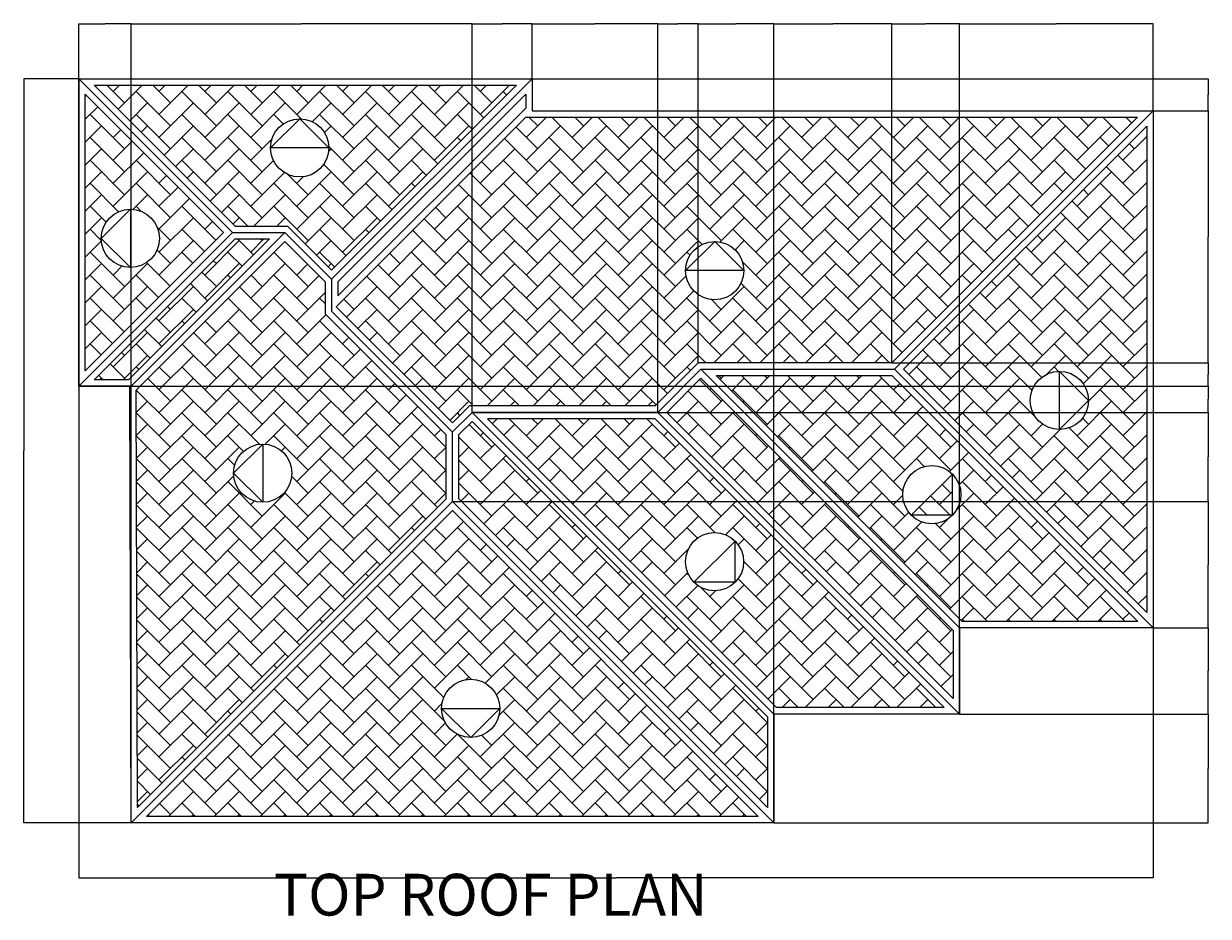
# Model space of a CAD drawing. Units: millimetres. Extents: x 19292 to 100733, y 12374 to 26974.
# Tile 23 of 24: x 60952 to 75784, y 12374 to 23551. Entities that reach past the tile are written whole.
import ezdxf

# ---------------------------------------------------------------- set-up
doc = ezdxf.new("R2010")
doc.units = ezdxf.units.MM
for name, color, linetype, lineweight in [('A-ANNO-DIMS', 2, 'Continuous', 18), ('A-ANNO-SYMB', 2, 'Continuous', 18), ('A-ANNO-TEXT', 7, 'Continuous', 35), ('A-ROOF', 6, 'Continuous', 25), ('A-ROOF-PATT', 8, 'Continuous', 13)]:
    doc.layers.add(name, color=color, linetype=linetype, lineweight=lineweight)
doc.styles.get("Standard").update_dxf_attribs({"font": 'arial.ttf'})
doc.dimstyles.get("Standard").update_dxf_attribs({"dimtxt": 0.18, "dimasz": 0.18, "dimexe": 0.18, "dimexo": 0.0625, "dimgap": 0.09, "dimtad": 0, "dimtih": 1, "dimtoh": 1, "dimdec": 4, "dimzin": 0, "dimdsep": 46, "dimtxsty": 'Standard', "dimcen": 0.09, "dimadec": 0, "dimazin": 0, "dimtfac": 1, "dimtdec": 4, "dimtofl": 0, "dimtmove": 0, "dimatfit": 3, "dimfxl": 1, "dimtolj": 1, "dimtzin": 0, "dimarcsym": 0})

# ---------------------------------------------------------------- blocks, each defined once
blk = doc.blocks.new('ROOF-SLOPE-SYMB')
for p, q in [((364.4880056519105, 728.9755004564394), (0.0002616674464662, 364.4877564719863)), ((364.4880056519105, 728.9755004564394), (728.9757496363599, 364.4877564719791)), ((728.9757496363673, 364.4877564719645), (0.0002616674464662, 364.4877564719863))]:
    blk.add_line(p, q)
blk.add_circle((364.4880056519032, 364.4877564719827), 364.4877439844593)
blk = doc.blocks.new('*D122')
at = {"layer": 'A-ANNO-DIMS', "color": 0, "lineweight": -2, "transparency": 16777216}
for p, q in [((61642.733569, 22860.787437), (61642.733569, 23550.904937)), ((61642.913569, 23550.724937), (61969.68047341132, 23550.724937)), ((62297.235768, 23550.724937), (61970.46886358869, 23550.724937)), ((62297.415768, 13544.0551), (62297.415768, 23550.904937))]:
    blk.add_line(p, q, dxfattribs=at)
at = {"layer": 'A-ANNO-DIMS', "color": 0, "transparency": 16777216}
for points in [[(61642.913569, 23550.754937), (61642.913569, 23550.694937), (61642.733569, 23550.724937)], [(62297.235768, 23550.754937), (62297.235768, 23550.694937), (62297.415768, 23550.724937)]]:
    blk.add_solid(points, dxfattribs=at)
at = {"layer": 'Defpoints', "color": 0, "transparency": 16777216}
for p in [(62297.415768, 23550.724937), (61642.733569, 22860.724937), (62297.415768, 13543.9926)]:
    blk.add_point(p, dxfattribs=at)
at = {"layer": 'A-ANNO-DIMS', "color": 0, "transparency": 16777216, "insert": (61970.0746685, 23550.724937), "char_height": 0.18, "attachment_point": 5}
blk.add_mtext('\\A1;654.7', dxfattribs=at)
blk = doc.blocks.new('*D123')
at = {"layer": 'A-ANNO-DIMS', "color": 0, "lineweight": -2, "transparency": 16777216}
for p, q in [((62297.415768, 13544.0551), (62297.415768, 23550.904937)), ((62297.595768, 23550.724937), (64431.20193955525, 23550.724937)), ((66565.53326800001, 23550.724937), (64431.92709644476, 23550.724937)), ((66565.713268, 18684.151922), (66565.713268, 23550.904937))]:
    blk.add_line(p, q, dxfattribs=at)
at = {"layer": 'A-ANNO-DIMS', "color": 0, "transparency": 16777216}
for points in [[(62297.595768, 23550.754937), (62297.595768, 23550.694937), (62297.415768, 23550.724937)], [(66565.53326800001, 23550.754937), (66565.53326800001, 23550.694937), (66565.713268, 23550.724937)]]:
    blk.add_solid(points, dxfattribs=at)
at = {"layer": 'Defpoints', "color": 0, "transparency": 16777216}
for p in [(66565.713268, 23550.724937), (66565.713268, 18684.089422), (62297.415768, 13543.9926)]:
    blk.add_point(p, dxfattribs=at)
at = {"layer": 'A-ANNO-DIMS', "color": 0, "transparency": 16777216, "insert": (64431.56451800001, 23550.724937), "char_height": 0.18, "attachment_point": 5}
blk.add_mtext('\\A1;4268', dxfattribs=at)
blk = doc.blocks.new('*D124')
at = {"layer": 'A-ANNO-DIMS', "color": 0, "lineweight": -2, "transparency": 16777216}
for p, q in [((66565.713268, 18684.151922), (66565.713268, 23550.904937)), ((66565.893268, 23550.724937), (66941.43622886836, 23550.724937)), ((67317.55356900001, 23550.724937), (66942.01060813166, 23550.724937)), ((67317.733569, 22860.787437), (67317.733569, 23550.904937))]:
    blk.add_line(p, q, dxfattribs=at)
at = {"layer": 'A-ANNO-DIMS', "color": 0, "transparency": 16777216}
for points in [[(66565.893268, 23550.754937), (66565.893268, 23550.694937), (66565.713268, 23550.724937)], [(67317.55356900001, 23550.754937), (67317.55356900001, 23550.694937), (67317.733569, 23550.724937)]]:
    blk.add_solid(points, dxfattribs=at)
at = {"layer": 'Defpoints', "color": 0, "transparency": 16777216}
for p in [(67317.733569, 23550.724937), (67317.733569, 22860.724937), (66565.713268, 18684.089422)]:
    blk.add_point(p, dxfattribs=at)
at = {"layer": 'A-ANNO-DIMS', "color": 0, "transparency": 16777216, "insert": (66941.72341850001, 23550.724937), "char_height": 0.18, "attachment_point": 5}
blk.add_mtext('\\A1;752', dxfattribs=at)
blk = doc.blocks.new('*D125')
at = {"layer": 'A-ANNO-DIMS', "color": 0, "lineweight": -2, "transparency": 16777216}
for p, q in [((67317.733569, 22860.787437), (67317.733569, 23550.904937)), ((67317.913569, 23550.724937), (68103.69878993586, 23550.724937)), ((68890.394693, 23550.724937), (68104.60947206413, 23550.724937)), ((68890.574693, 18684.151922), (68890.574693, 23550.904937))]:
    blk.add_line(p, q, dxfattribs=at)
at = {"layer": 'A-ANNO-DIMS', "color": 0, "transparency": 16777216}
for points in [[(67317.913569, 23550.754937), (67317.913569, 23550.694937), (67317.733569, 23550.724937)], [(68890.394693, 23550.754937), (68890.394693, 23550.694937), (68890.574693, 23550.724937)]]:
    blk.add_solid(points, dxfattribs=at)
at = {"layer": 'Defpoints', "color": 0, "transparency": 16777216}
for p in [(68890.574693, 23550.724937), (67317.733569, 22860.724937), (68890.574693, 18684.089422)]:
    blk.add_point(p, dxfattribs=at)
at = {"layer": 'A-ANNO-DIMS', "color": 0, "transparency": 16777216, "insert": (68104.154131, 23550.724937), "char_height": 0.18, "attachment_point": 5}
blk.add_mtext('\\A1;1572.8', dxfattribs=at)
blk = doc.blocks.new('*D126')
at = {"layer": 'A-ANNO-DIMS', "color": 0, "lineweight": -2, "transparency": 16777216}
for p, q in [((68890.574693, 18684.151922), (68890.574693, 23550.904937)), ((68890.754693, 23550.724937), (69143.34455204367, 23550.724937)), ((69396.72181900001, 23550.724937), (69144.13195995636, 23550.724937)), ((69396.901819, 19303.616133), (69396.901819, 23550.904937))]:
    blk.add_line(p, q, dxfattribs=at)
at = {"layer": 'A-ANNO-DIMS', "color": 0, "transparency": 16777216}
for points in [[(68890.754693, 23550.754937), (68890.754693, 23550.694937), (68890.574693, 23550.724937)], [(69396.72181900001, 23550.754937), (69396.72181900001, 23550.694937), (69396.901819, 23550.724937)]]:
    blk.add_solid(points, dxfattribs=at)
at = {"layer": 'Defpoints', "color": 0, "transparency": 16777216}
for p in [(69396.901819, 23550.724937), (69396.901819, 19303.553633), (68890.574693, 18684.089422)]:
    blk.add_point(p, dxfattribs=at)
at = {"layer": 'A-ANNO-DIMS', "color": 0, "transparency": 16777216, "insert": (69143.73825600001, 23550.724937), "char_height": 0.18, "attachment_point": 5}
blk.add_mtext('\\A1;506.3', dxfattribs=at)
blk = doc.blocks.new('*D127')
at = {"layer": 'A-ANNO-DIMS', "color": 0, "lineweight": -2, "transparency": 16777216}
for p, q in [((69396.901819, 19303.616133), (69396.901819, 23550.904937)), ((69397.081819, 23550.724937), (69869.75634673669, 23550.724937)), ((70343.219633, 23550.724937), (69870.5451052633, 23550.724937)), ((70343.399633, 13544.0551), (70343.399633, 23550.904937))]:
    blk.add_line(p, q, dxfattribs=at)
at = {"layer": 'A-ANNO-DIMS', "color": 0, "transparency": 16777216}
for points in [[(69397.081819, 23550.754937), (69397.081819, 23550.694937), (69396.901819, 23550.724937)], [(70343.219633, 23550.754937), (70343.219633, 23550.694937), (70343.399633, 23550.724937)]]:
    blk.add_solid(points, dxfattribs=at)
at = {"layer": 'Defpoints', "color": 0, "transparency": 16777216}
for p in [(70343.399633, 23550.724937), (69396.901819, 19303.553633), (70343.399633, 13543.9926)]:
    blk.add_point(p, dxfattribs=at)
at = {"layer": 'A-ANNO-DIMS', "color": 0, "transparency": 16777216, "insert": (69870.15072599999, 23550.724937), "char_height": 0.18, "attachment_point": 5}
blk.add_mtext('\\A1;946.5', dxfattribs=at)
blk = doc.blocks.new('*D128')
at = {"layer": 'A-ANNO-DIMS', "color": 0, "lineweight": -2, "transparency": 16777216}
for p, q in [((70343.399633, 13544.0551), (70343.399633, 23550.904937)), ((70343.57963299999, 23550.724937), (71082.56192218894, 23550.724937)), ((71822.24518000001, 23550.724937), (71083.26289081105, 23550.724937)), ((71822.42518, 19303.616133), (71822.42518, 23550.904937))]:
    blk.add_line(p, q, dxfattribs=at)
at = {"layer": 'A-ANNO-DIMS', "color": 0, "transparency": 16777216}
for points in [[(70343.57963299999, 23550.754937), (70343.57963299999, 23550.694937), (70343.399633, 23550.724937)], [(71822.24518000001, 23550.754937), (71822.24518000001, 23550.694937), (71822.42518, 23550.724937)]]:
    blk.add_solid(points, dxfattribs=at)
at = {"layer": 'Defpoints', "color": 0, "transparency": 16777216}
for p in [(71822.42518, 23550.724937), (71822.42518, 19303.553633), (70343.399633, 13543.9926)]:
    blk.add_point(p, dxfattribs=at)
at = {"layer": 'A-ANNO-DIMS', "color": 0, "transparency": 16777216, "insert": (71082.91240649999, 23550.724937), "char_height": 0.18, "attachment_point": 5}
blk.add_mtext('\\A1;1479', dxfattribs=at)
blk = doc.blocks.new('*D129')
at = {"layer": 'A-ANNO-DIMS', "color": 0, "lineweight": -2, "transparency": 16777216}
for p, q in [((71822.42518, 19303.616133), (71822.42518, 23550.904937)), ((71822.60518, 23550.724937), (72244.94910808594, 23550.724937)), ((72668.08105800001, 23550.724937), (72245.73712991405, 23550.724937)), ((72668.261058, 14906.465557), (72668.261058, 23550.904937))]:
    blk.add_line(p, q, dxfattribs=at)
at = {"layer": 'A-ANNO-DIMS', "color": 0, "transparency": 16777216}
for points in [[(71822.60518, 23550.754937), (71822.60518, 23550.694937), (71822.42518, 23550.724937)], [(72668.08105800001, 23550.754937), (72668.08105800001, 23550.694937), (72668.261058, 23550.724937)]]:
    blk.add_solid(points, dxfattribs=at)
at = {"layer": 'Defpoints', "color": 0, "transparency": 16777216}
for p in [(72668.261058, 23550.724937), (71822.42518, 19303.553633), (72668.261058, 14906.403057)]:
    blk.add_point(p, dxfattribs=at)
at = {"layer": 'A-ANNO-DIMS', "color": 0, "transparency": 16777216, "insert": (72245.343119, 23550.724937), "char_height": 0.18, "attachment_point": 5}
blk.add_mtext('\\A1;845.8', dxfattribs=at)
blk = doc.blocks.new('*D130')
at = {"layer": 'A-ANNO-DIMS', "color": 0, "lineweight": -2, "transparency": 16777216}
for p, q in [((72668.261058, 14906.465557), (72668.261058, 23550.904937)), ((72668.441058, 23550.724937), (73880.03147448227, 23550.724937)), ((75092.55356900001, 23550.724937), (73880.96315251774, 23550.724937)), ((75092.733569, 22460.787437), (75092.733569, 23550.904937))]:
    blk.add_line(p, q, dxfattribs=at)
at = {"layer": 'A-ANNO-DIMS', "color": 0, "transparency": 16777216}
for points in [[(72668.441058, 23550.754937), (72668.441058, 23550.694937), (72668.261058, 23550.724937)], [(75092.55356900001, 23550.754937), (75092.55356900001, 23550.694937), (75092.733569, 23550.724937)]]:
    blk.add_solid(points, dxfattribs=at)
at = {"layer": 'Defpoints', "color": 0, "transparency": 16777216}
for p in [(75092.733569, 23550.724937), (75092.733569, 22460.724937), (72668.261058, 14906.403057)]:
    blk.add_point(p, dxfattribs=at)
at = {"layer": 'A-ANNO-DIMS', "color": 0, "transparency": 16777216, "insert": (73880.4973135, 23550.724937), "char_height": 0.18, "attachment_point": 5}
blk.add_mtext('\\A1;2424.5', dxfattribs=at)
blk = doc.blocks.new('*D131')
at = {"layer": 'A-ANNO-DIMS', "color": 0, "lineweight": -2, "transparency": 16777216}
for p, q in [((72668.32355800003, 14906.40305700001), (75783.96435500005, 14906.40305700001)), ((75783.78435500005, 14906.223057), (75783.78435500005, 14225.37979302934)), ((75783.78435500005, 13544.17260000001), (75783.78435500005, 14225.01586397067)), ((70343.46213300002, 13543.9926), (75783.96435500005, 13543.9926))]:
    blk.add_line(p, q, dxfattribs=at)
at = {"layer": 'A-ANNO-DIMS', "color": 0, "transparency": 16777216}
for points in [[(75783.75435500006, 14906.223057), (75783.81435500005, 14906.223057), (75783.78435500005, 14906.40305700001)], [(75783.75435500006, 13544.17260000001), (75783.81435500005, 13544.17260000001), (75783.78435500005, 13543.9926)]]:
    blk.add_solid(points, dxfattribs=at)
at = {"layer": 'Defpoints', "color": 0, "transparency": 16777216}
for p in [(72668.26105800003, 14906.40305700001), (75783.78435500005, 14906.40305700001), (70343.39963300002, 13543.9926)]:
    blk.add_point(p, dxfattribs=at)
at = {"layer": 'A-ANNO-DIMS', "color": 0, "transparency": 16777216, "insert": (75783.78435500004, 14225.19782849998), "char_height": 0.18, "attachment_point": 5}
blk.add_mtext('\\A1;1362.4', dxfattribs=at)
blk = doc.blocks.new('*D132')
at = {"layer": 'A-ANNO-DIMS', "color": 0, "lineweight": -2, "transparency": 16777216}
for p, q in [((75093.84685500003, 15985.72510100001), (75783.96435500005, 15985.72510100001)), ((75783.78435500005, 15985.545101), (75783.78435500005, 15446.24604352934)), ((75783.78435500005, 14906.583057), (75783.78435500005, 15445.88211447067)), ((72668.32355800003, 14906.40305700001), (75783.96435500005, 14906.40305700001))]:
    blk.add_line(p, q, dxfattribs=at)
at = {"layer": 'A-ANNO-DIMS', "color": 0, "transparency": 16777216}
for points in [[(75783.75435500006, 15985.545101), (75783.81435500005, 15985.545101), (75783.78435500005, 15985.72510100001)], [(75783.75435500006, 14906.583057), (75783.81435500005, 14906.583057), (75783.78435500005, 14906.40305700001)]]:
    blk.add_solid(points, dxfattribs=at)
at = {"layer": 'Defpoints', "color": 0, "transparency": 16777216}
for p in [(75093.78435500003, 15985.72510100001), (75783.78435500005, 15985.72510100001), (72668.26105800003, 14906.40305700001)]:
    blk.add_point(p, dxfattribs=at)
at = {"layer": 'A-ANNO-DIMS', "color": 0, "transparency": 16777216, "insert": (75783.78435500004, 15446.06407899998), "char_height": 0.18, "attachment_point": 5}
blk.add_mtext('\\A1;1079.3', dxfattribs=at)
blk = doc.blocks.new('*D133')
at = {"layer": 'A-ANNO-DIMS', "color": 0, "lineweight": -2, "transparency": 16777216}
for p, q in [((66320.47020100003, 17566.98453300001), (75783.96435500005, 17566.98453300001)), ((75783.78435500005, 17566.80453300001), (75783.78435500005, 16776.53678152934)), ((75783.78435500005, 15985.90510100001), (75783.78435500005, 16776.17285247068)), ((75093.84685500003, 15985.72510100001), (75783.96435500005, 15985.72510100001))]:
    blk.add_line(p, q, dxfattribs=at)
at = {"layer": 'A-ANNO-DIMS', "color": 0, "transparency": 16777216}
for points in [[(75783.75435500006, 17566.80453300001), (75783.81435500005, 17566.80453300001), (75783.78435500005, 17566.98453300001)], [(75783.75435500006, 15985.90510100001), (75783.81435500005, 15985.90510100001), (75783.78435500005, 15985.72510100001)]]:
    blk.add_solid(points, dxfattribs=at)
at = {"layer": 'Defpoints', "color": 0, "transparency": 16777216}
for p in [(66320.40770100003, 17566.98453300001), (75783.78435500005, 17566.98453300001), (75093.78435500003, 15985.72510100001)]:
    blk.add_point(p, dxfattribs=at)
at = {"layer": 'A-ANNO-DIMS', "color": 0, "transparency": 16777216, "insert": (75783.78435500004, 16776.35481699998), "char_height": 0.18, "attachment_point": 5}
blk.add_mtext('\\A1;1581.3', dxfattribs=at)
blk = doc.blocks.new('*D134')
at = {"layer": 'A-ANNO-DIMS', "color": 0, "lineweight": -2, "transparency": 16777216}
for p, q in [((66565.77576800004, 18684.08942200001), (75783.96435500005, 18684.08942200001)), ((75783.78435500005, 18683.90942200001), (75783.78435500005, 18125.71734584926)), ((75783.78435500005, 17567.16453300001), (75783.78435500005, 18125.35660915076)), ((66320.47020100003, 17566.98453300001), (75783.96435500005, 17566.98453300001))]:
    blk.add_line(p, q, dxfattribs=at)
at = {"layer": 'A-ANNO-DIMS', "color": 0, "transparency": 16777216}
for points in [[(75783.75435500006, 18683.90942200001), (75783.81435500005, 18683.90942200001), (75783.78435500005, 18684.08942200001)], [(75783.75435500006, 17567.16453300001), (75783.81435500005, 17567.16453300001), (75783.78435500005, 17566.98453300001)]]:
    blk.add_solid(points, dxfattribs=at)
at = {"layer": 'Defpoints', "color": 0, "transparency": 16777216}
for p in [(66565.71326800004, 18684.08942200001), (75783.78435500005, 18684.08942200001), (66320.40770100003, 17566.98453300001)]:
    blk.add_point(p, dxfattribs=at)
at = {"layer": 'A-ANNO-DIMS', "color": 0, "transparency": 16777216, "insert": (75783.78435500004, 18125.53697749998), "char_height": 0.18, "attachment_point": 5}
blk.add_mtext('\\A1;1117', dxfattribs=at)
blk = doc.blocks.new('*D135')
at = {"layer": 'A-ANNO-DIMS', "color": 0, "lineweight": -2, "transparency": 16777216}
for p, q in [((61642.79606900003, 19010.724937), (75783.96435500005, 19010.72493700001)), ((75783.78435500005, 19010.54493700001), (75783.78435500005, 18847.58914402934)), ((75783.78435500005, 18684.26942200001), (75783.78435500005, 18847.22521497068)), ((66565.77576800004, 18684.08942200001), (75783.96435500005, 18684.08942200001))]:
    blk.add_line(p, q, dxfattribs=at)
at = {"layer": 'A-ANNO-DIMS', "color": 0, "transparency": 16777216}
for points in [[(75783.75435500006, 19010.54493700001), (75783.81435500005, 19010.54493700001), (75783.78435500005, 19010.72493700001)], [(75783.75435500006, 18684.26942200001), (75783.81435500005, 18684.26942200001), (75783.78435500005, 18684.08942200001)]]:
    blk.add_solid(points, dxfattribs=at)
at = {"layer": 'Defpoints', "color": 0, "transparency": 16777216}
for p in [(61642.73356900003, 19010.724937), (75783.78435500005, 19010.72493700001), (66565.71326800004, 18684.08942200001)]:
    blk.add_point(p, dxfattribs=at)
at = {"layer": 'A-ANNO-DIMS', "color": 0, "transparency": 16777216, "insert": (75783.78435500004, 18847.40717949999), "char_height": 0.18, "attachment_point": 5}
blk.add_mtext('\\A1;326.64', dxfattribs=at)
blk = doc.blocks.new('*D136')
at = {"layer": 'A-ANNO-DIMS', "color": 0, "lineweight": -2, "transparency": 16777216}
for p, q in [((71822.48768000003, 19303.55363300001), (75783.96435500005, 19303.55363300001)), ((75783.78435500005, 19303.37363300001), (75783.78435500005, 19157.3211881378)), ((75783.78435500005, 19010.90493700001), (75783.78435500005, 19156.95738186222)), ((61642.79606900003, 19010.724937), (75783.96435500005, 19010.72493700001))]:
    blk.add_line(p, q, dxfattribs=at)
at = {"layer": 'A-ANNO-DIMS', "color": 0, "transparency": 16777216}
for points in [[(75783.75435500006, 19303.37363300001), (75783.81435500005, 19303.37363300001), (75783.78435500005, 19303.55363300001)], [(75783.75435500006, 19010.90493700001), (75783.81435500005, 19010.90493700001), (75783.78435500005, 19010.72493700001)]]:
    blk.add_solid(points, dxfattribs=at)
at = {"layer": 'Defpoints', "color": 0, "transparency": 16777216}
for p in [(71822.42518000003, 19303.55363300001), (75783.78435500005, 19303.55363300001), (61642.73356900003, 19010.724937)]:
    blk.add_point(p, dxfattribs=at)
at = {"layer": 'A-ANNO-DIMS', "color": 0, "transparency": 16777216, "insert": (75783.78435500004, 19157.13928499998), "char_height": 0.18, "attachment_point": 5}
blk.add_mtext('\\A1;292.8', dxfattribs=at)
blk = doc.blocks.new('*D137')
at = {"layer": 'A-ANNO-DIMS', "color": 0, "lineweight": -2, "transparency": 16777216}
for p, q in [((75092.79606900003, 22460.72493700001), (75783.96435500005, 22460.72493700001)), ((75783.78435500005, 22460.54493700001), (75783.78435500005, 20882.32124952934)), ((75783.78435500005, 19303.73363300001), (75783.78435500005, 20881.95732047068)), ((71822.48768000003, 19303.55363300001), (75783.96435500005, 19303.55363300001))]:
    blk.add_line(p, q, dxfattribs=at)
at = {"layer": 'A-ANNO-DIMS', "color": 0, "transparency": 16777216}
for points in [[(75783.75435500006, 22460.54493700001), (75783.81435500005, 22460.54493700001), (75783.78435500005, 22460.72493700001)], [(75783.75435500006, 19303.73363300001), (75783.81435500005, 19303.73363300001), (75783.78435500005, 19303.55363300001)]]:
    blk.add_solid(points, dxfattribs=at)
at = {"layer": 'Defpoints', "color": 0, "transparency": 16777216}
for p in [(75092.73356900003, 22460.72493700001), (75783.78435500005, 22460.72493700001), (71822.42518000003, 19303.55363300001)]:
    blk.add_point(p, dxfattribs=at)
at = {"layer": 'A-ANNO-DIMS', "color": 0, "transparency": 16777216, "insert": (75783.78435500004, 20882.13928499998), "char_height": 0.18, "attachment_point": 5}
blk.add_mtext('\\A1;3157', dxfattribs=at)
blk = doc.blocks.new('*D138')
at = {"layer": 'A-ANNO-DIMS', "color": 0, "lineweight": -2, "transparency": 16777216}
for p, q in [((67317.79606900003, 22860.72493700001), (75783.96435500005, 22860.72493700001)), ((75783.78435500005, 22860.54493700001), (75783.78435500005, 22660.90684013779)), ((75783.78435500005, 22460.90493700001), (75783.78435500005, 22660.54303386222)), ((75092.79606900003, 22460.72493700001), (75783.96435500005, 22460.72493700001))]:
    blk.add_line(p, q, dxfattribs=at)
at = {"layer": 'A-ANNO-DIMS', "color": 0, "transparency": 16777216}
for points in [[(75783.75435500006, 22860.54493700001), (75783.81435500005, 22860.54493700001), (75783.78435500005, 22860.72493700001)], [(75783.75435500006, 22460.90493700001), (75783.81435500005, 22460.90493700001), (75783.78435500005, 22460.72493700001)]]:
    blk.add_solid(points, dxfattribs=at)
at = {"layer": 'Defpoints', "color": 0, "transparency": 16777216}
for p in [(67317.73356900003, 22860.72493700001), (75783.78435500005, 22860.72493700001), (75092.73356900003, 22460.72493700001)]:
    blk.add_point(p, dxfattribs=at)
at = {"layer": 'A-ANNO-DIMS', "color": 0, "transparency": 16777216, "insert": (75783.78435500004, 22660.72493699998), "char_height": 0.18, "attachment_point": 5}
blk.add_mtext('\\A1;400', dxfattribs=at)
blk = doc.blocks.new('*D139')
at = {"layer": 'A-ANNO-DIMS', "color": 0, "lineweight": -2, "transparency": 16777216}
for p, q in [((61642.733569, 22860.662437), (61642.733569, 12853.8126)), ((75093.784355, 15985.662601), (75093.784355, 12853.8126)), ((61642.913569, 12853.9926), (68367.85611070396, 12853.9926)), ((75093.604355, 12853.9926), (68368.66181329606, 12853.9926))]:
    blk.add_line(p, q, dxfattribs=at)
at = {"layer": 'A-ANNO-DIMS', "color": 0, "transparency": 16777216}
for points in [[(61642.913569, 12854.0226), (61642.913569, 12853.9626), (61642.733569, 12853.9926)], [(75093.604355, 12854.0226), (75093.604355, 12853.9626), (75093.784355, 12853.9926)]]:
    blk.add_solid(points, dxfattribs=at)
at = {"layer": 'Defpoints', "color": 0, "transparency": 16777216}
for p in [(61642.733569, 22860.724937), (75093.784355, 15985.725101), (75093.784355, 12853.9926)]:
    blk.add_point(p, dxfattribs=at)
at = {"layer": 'A-ANNO-DIMS', "color": 0, "transparency": 16777216, "insert": (68368.258962, 12853.9926), "char_height": 0.18, "attachment_point": 5}
blk.add_mtext('\\A1;13451', dxfattribs=at)
blk = doc.blocks.new('*D140')
at = {"layer": 'A-ANNO-DIMS', "color": 0, "lineweight": -2, "transparency": 16777216}
for p, q in [((61642.67106900003, 22860.72493700001), (60952.55356900006, 22860.72493700001)), ((60952.73356900006, 22860.54493700001), (60952.73356900006, 18202.54073302934)), ((60952.73356900007, 13544.1726), (60952.73356900006, 18202.17680397067)), ((62297.35326800002, 13543.9926), (60952.55356900007, 13543.9926))]:
    blk.add_line(p, q, dxfattribs=at)
at = {"layer": 'A-ANNO-DIMS', "color": 0, "transparency": 16777216}
for points in [[(60952.70356900006, 22860.54493700001), (60952.76356900006, 22860.54493700001), (60952.73356900006, 22860.72493700001)], [(60952.70356900007, 13544.1726), (60952.76356900007, 13544.1726), (60952.73356900007, 13543.9926)]]:
    blk.add_solid(points, dxfattribs=at)
at = {"layer": 'Defpoints', "color": 0, "transparency": 16777216}
for p in [(61642.73356900003, 22860.72493700001), (60952.73356900007, 13543.9926), (62297.41576800003, 13543.9926)]:
    blk.add_point(p, dxfattribs=at)
at = {"layer": 'A-ANNO-DIMS', "color": 0, "transparency": 16777216, "insert": (60952.73356900006, 18202.35876849998), "char_height": 0.18, "attachment_point": 5}
blk.add_mtext('\\A1;9317', dxfattribs=at)

msp = doc.modelspace()

# ---------------------------------------------------------------- hatches: boundary and pattern name
at = {"layer": 'A-ROOF-PATT'}
h = msp.add_hatch(dxfattribs=at)
h.set_pattern_fill('AR-HBONE', color=256, scale=2)
h.set_pattern_definition([(45, (0, 0), (0, 287.3681958742129), [609.6, -203.2]), (135, (143.684, 143.684), (2.84e-14, 287.3681958742129), [609.6, -203.2])])
h.paths.add_polyline_path([(64727.08205220358, 19916.93633462452), (64727.08205220358, 20316.93633462452), (64221.43053501982, 20822.58785180828), (62360.67751289125, 18961.8348296797), (62376.82128203092, 13736.5351991242), (66240.40770068225, 17600.12161777552), (66240.40770068225, 18403.61068614586)])
h.paths.add_polyline_path([(64310.17877957573, 17922.72950283403, -1), (63581.20329160683, 17922.72950283403, -1)], flags=16)
h.paths.add_polyline_path([(63945.69103559129, 18287.21724681849), (63945.69103559128, 17558.24175884957), (63581.20329160683, 17922.72950283402)], flags=0)
h.paths.add_polyline_path([(64028.29345002997, 20855.72493679813), (63600.87065437719, 20855.72493679813), (61836.46959126122, 19091.32387368216), (62265.21701898907, 19092.64850575723)])
h.paths.add_polyline_path([(67124.59648439751, 22780.72493679813), (61835.87065437719, 22780.72493679813), (63600.8706543772, 21015.72493679813), (64254.56762000968, 21015.72493679813), (64807.08205220358, 20463.21050460422)])
h.paths.add_polyline_path([(64773.07274963637, 21996.07375647198, -1), (64044.09726166745, 21996.07375647198, -1)], flags=16)
h.paths.add_polyline_path([(64044.09726166745, 21996.07375647198), (64408.58500565191, 22360.56150045644), (64773.07274963638, 21996.07375647197)], flags=0)
h.paths.add_polyline_path([(61722.73356938735, 22667.58785180828), (61722.73356938735, 19203.86202178798), (63454.5964843975, 20935.72493679813)])
h.paths.add_polyline_path([(62652.72125307563, 20862.10236338188, -1), (61923.74576510673, 20862.10236338188, -1)], flags=16)
h.paths.add_polyline_path([(62288.23350909119, 21226.59010736635), (62288.23350909117, 20497.61461939743), (61923.74576510673, 20862.10236338188)], flags=0)
h.paths.add_polyline_path([(74899.59648439751, 22380.72493679813), (67237.73356938735, 22380.72493679813), (64863.65059469851, 20006.6419621093), (66319.38965928082, 18550.90289752698), (66532.57618349593, 18764.08942174208), (68857.43760794727, 18764.08942174208), (69396.9018188986, 19303.5536326934), (71822.42518029278, 19303.5536326934)])
h.paths.add_polyline_path([(69969.42866692018, 20459.2445118836, -1), (69240.45317895127, 20459.2445118836, -1)], flags=16)
h.paths.add_polyline_path([(69240.45317895127, 20459.2445118836), (69604.94092293573, 20823.73225586806), (69969.42866692018, 20459.24451188359)], flags=0)
h.paths.add_polyline_path([(75012.76490621475, 22267.61918863569), (71968.89612956435, 19223.75041198531), (75013.75300605538, 16178.89353549429)])
h.paths.add_polyline_path([(74284.79238763452, 18832.89103207015, -1), (73555.8168996656, 18832.89103207015, -1)], flags=16)
h.paths.add_polyline_path([(73920.30464365006, 19197.37877605462), (74284.79238763452, 18832.89103207016), (73920.30464365004, 18468.40328808569)], flags=0)
h.paths.add_polyline_path([(71822.8187388766, 19143.5536326934), (69623.17598887825, 19143.5536326934), (72701.39276485311, 16065.33685671856), (74900.67860700011, 16065.69376456988)])
h.paths.add_polyline_path([(72687.06251920365, 17654.15776277031, -1), (71958.08703123474, 17654.15776277031, -1)], flags=16)
h.paths.add_polyline_path([(72580.30653064999, 17911.8895182011), (72580.30653064999, 17396.42600733951), (72064.84301978839, 17396.42600733952)], flags=16)
h.paths.add_polyline_path([(69430.03890388843, 19110.41654770356), (69003.71177792695, 18684.08942174208), (72588.26105764683, 15099.5401420222), (72588.26105764683, 15952.19439394516)])
h.paths.add_polyline_path([(68857.43760794726, 18604.08942174208), (66758.8503534756, 18604.08942174208), (70376.53671818532, 14986.40305703235), (72475.12397265699, 14986.40305703235)])
h.paths.add_polyline_path([(69966.34480153024, 16814.40136553731, -1), (69237.36931356133, 16814.40136553731, -1)], flags=16)
h.paths.add_polyline_path([(69859.58881297658, 17072.13312096811), (69859.58881297658, 16556.66961010652), (69344.12530211498, 16556.66961010653)], flags=0)
h.paths.add_polyline_path([(66565.71326848576, 18570.95233675224), (66400.40770068225, 18405.64676894872), (66400.40770068225, 17600.12161777552), (70263.39963319548, 13737.12968526228), (70263.39963319548, 14873.26597204251)])
h.paths.add_polyline_path([(66320.40770068225, 17453.84744779584), (62490.55285315886, 13623.99260027244), (70150.26254820565, 13623.99260027244)])
h.paths.add_polyline_path([(66913.53751657206, 14976.74606750543, -1), (66184.56202860315, 14976.74606750543, -1)], flags=16)
h.paths.add_polyline_path([(66184.56202860315, 14976.74606750544), (66913.53751657206, 14976.74606750544), (66549.04977258762, 14612.25832352097)], flags=0)

# ---------------------------------------------------------------- linework, layer by layer
at = {"layer": 'A-ROOF'}
for p, q in [((61642.73356938735, 22860.72493679813), (63567.73356938735, 20935.72493679813)), ((64807.08205220358, 20350.07341961437), (67317.73356938735, 22860.72493679813)), ((61642.73356938735, 19010.72493679813), (63567.73356938735, 20935.72493679813)), ((62280.57506925564, 18994.86947103394), (64221.43053501982, 20935.72493679813)), ((63567.73356938735, 20935.72493679813), (64221.43053501982, 20935.72493679813)), ((63600.87065437719, 21015.72493679813), (64254.56762000968, 21015.72493679813)), ((64221.43053501982, 20935.72493679813), (64807.08205220358, 20350.07341961437)), ((64254.56762000968, 21015.72493679813), (64807.08205220358, 20463.21050460422)), ((63600.87065437719, 20855.72493679813), (64028.29345002997, 20855.72493679813)), ((64221.43053501982, 20822.58785180828), (64727.08205220358, 20316.93633462452)), ((64807.08205220358, 20350.07341961437), (64807.08205220358, 19950.07341961437)), ((64727.08205220358, 20316.93633462452), (64727.08205220358, 19916.93633462452)), ((64887.08205220358, 20316.93633462452), (64887.08205220358, 20143.21050460422)), ((64727.08205220358, 19916.93633462452), (66240.40770068225, 18403.61068614586)), ((64807.08205220358, 19950.07341961437), (66319.38965928082, 18437.76581253714)), ((64863.65059469851, 20006.6419621093), (66319.38965928082, 18550.90289752698)), ((69396.9018188986, 19303.5536326934), (68857.43760794727, 18764.08942174208)), ((71822.42518029278, 19303.5536326934), (69396.9018188986, 19303.5536326934)), ((69430.03890388843, 19223.5536326934), (68890.57469293711, 18684.08942174208)), ((69430.03890388843, 19110.41654770356), (69003.71177792695, 18684.08942174208)), ((66532.57618349593, 18764.08942174208), (66319.38965928082, 18550.90289752697)), ((68857.43760794727, 18764.08942174208), (66532.57618349593, 18764.08942174208)), ((66565.71326848576, 18684.08942174208), (66320.40770068225, 18438.78385393857)), ((66565.71326848576, 18570.95233675224), (66400.40770068225, 18405.64676894872)), ((66565.71326848576, 18684.08942174208), (70343.39963319548, 14906.40305703235)), ((68890.57469293711, 18684.08942174208), (66565.71326848576, 18684.08942174208)), ((68857.43760794726, 18604.08942174208), (66758.8503534756, 18604.08942174208)), ((68890.57469293711, 18684.08942174208), (72668.26105764683, 14906.40305703235)), ((66240.40770068225, 17600.12161777552), (66240.40770068225, 18403.61068614586)), ((66320.40770068225, 17566.98453278568), (66320.40770068225, 18438.78385393857)), ((66400.40770068225, 17600.12161777552), (66400.40770068225, 18405.64676894872)), ((62297.41576816901, 13543.99260027244), (66320.40770068225, 17566.98453278568)), ((66320.40770068225, 17566.98453278568), (70343.39963319548, 13543.99260027244))]:
    msp.add_line(p, q, dxfattribs=at)
for points in [[(61642.73356938735, 22860.72493679813), (67317.73356938735, 22860.72493679813), (67317.73356938735, 22460.72493679813), (75092.73356938735, 22460.72493679813), (75093.78435516256, 15985.72510139728), (72668.26105764683, 15985.331478935), (72668.26105764683, 14906.40305703235), (70343.39963319548, 14906.40305703235), (70343.39963319548, 13543.99260027244), (62297.41576816901, 13543.99260027244), (62280.519995336, 19012.69540309651), (61642.73356938735, 19010.72493679813), (61642.73356938735, 22860.72493679813)], [(63600.87065437719, 21015.72493679813), (61835.87065437719, 22780.72493679813), (67124.59648439751, 22780.72493679813), (64807.08205220358, 20463.21050460422)], [(63454.59648439749, 20935.72493679813), (61722.73356938735, 19203.86202178798), (61722.73356938735, 22667.58785180828), (63454.59648439749, 20935.72493679813)], [(64887.08205220358, 20316.93633462452), (67237.73356938735, 22667.58785180829), (67237.73356938735, 22493.86202178797), (64887.08205220358, 20143.21050460422)], [(75092.73356938735, 22460.72493679813), (71855.75904457452, 19223.75041198531), (75093.78435516256, 15985.72510139728), (72668.26105764683, 15985.331478935), (69430.03890388843, 19223.5536326934), (71855.95582386643, 19223.5536326934)], [(64863.65059469851, 20006.6419621093), (67237.73356938735, 22380.72493679813), (74899.59648439751, 22380.72493679813), (71822.42518029278, 19303.5536326934)], [(71968.89612956435, 19223.75041198531), (75012.76490621475, 22267.61918863569), (75013.75300605538, 16178.89353549429), (71968.89612956435, 19223.75041198531)], [(64028.29345002997, 20855.72493679813), (62265.21701898907, 19092.64850575723), (61836.46959126122, 19091.32387368216), (63600.87065437719, 20855.72493679813)], [(66240.40770068225, 17600.12161777552), (62376.82128203092, 13736.5351991242), (62360.67751289125, 18961.8348296797), (64221.43053501982, 20822.58785180828)], [(71822.8187388766, 19143.5536326934), (74900.67860700011, 16065.69376456988), (72701.39276485311, 16065.33685671856), (69623.17598887825, 19143.5536326934), (71822.8187388766, 19143.5536326934)], [(69430.03890388843, 19110.41654770356), (72588.26105764683, 15952.19439394516), (72588.26105764683, 15099.5401420222), (69003.71177792695, 18684.08942174208)], [(66565.71326848576, 18570.95233675224), (70263.39963319548, 14873.26597204251), (70263.39963319548, 13737.12968526228), (66400.40770068225, 17600.12161777552)], [(68857.43760794726, 18604.08942174208), (72475.12397265699, 14986.40305703235), (70376.53671818532, 14986.40305703235), (66758.8503534756, 18604.08942174208)], [(70150.26254820565, 13623.99260027244), (62490.55285315886, 13623.99260027244), (66320.40770068225, 17453.84744779584), (70150.26254820565, 13623.99260027244)]]:
    msp.add_lwpolyline(points, dxfattribs=at)

# ---------------------------------------------------------------- block references
at = {"layer": 'A-ANNO-SYMB'}
for p in [(64044.09700000001, 21631.586), (69240.45291728381, 20094.75675541162)]:
    msp.add_blockref('ROOF-SLOPE-SYMB', p, dxfattribs=at)
for p, rotation in [((62652.72126556317, 20497.61435772999), 90.00000000000175), ((73555.8168871781, 19197.37903772207), 269.9999999999988), ((64310.17879206329, 17558.24149718212), 90.00000000000202), ((72322.57495141604, 18169.62146748874), 224.9999999999987), ((69601.85723374262, 17329.86507025575), 224.9999999999988), ((66913.53777823951, 15341.23382397741), 180)]:
    msp.add_blockref('ROOF-SLOPE-SYMB', p, dxfattribs=dict(at, rotation=rotation))

# ---------------------------------------------------------------- texts
at = {"layer": 'A-ANNO-TEXT'}
msp.add_text('TOP ROOF PLAN', height=523.2684807306957, dxfattribs=at).set_placement((64086.89395526097, 12383.03142158251))

# ---------------------------------------------------------------- dimensions: what is measured, and where the dimension line sits
at = {"layer": 'A-ANNO-DIMS'}
for base, p1, p2, override, picture, middle in [((62297.415768, 23550.724937), (61642.733569, 22860.724937), (62297.415768, 13543.9926), {"dimdec": 1, "dimlfac": 1, "dimrnd": 0, "dimzin": 0, "dimdsep": 46, "dimlunit": 2}, '*D122', (61970.0746685, 23550.724937)), ((66565.713268, 23550.724937), (62297.415768, 13543.9926), (66565.713268, 18684.089422), {"dimdec": 0, "dimlfac": 1, "dimrnd": 0, "dimzin": 0, "dimdsep": 46, "dimlunit": 2}, '*D123', (64431.56451800001, 23550.724937)), ((67317.733569, 23550.724937), (66565.713268, 18684.089422), (67317.733569, 22860.724937), {"dimdec": 0, "dimlfac": 1, "dimrnd": 0, "dimzin": 0, "dimdsep": 46, "dimlunit": 2}, '*D124', (66941.72341850001, 23550.724937)), ((68890.574693, 23550.724937), (67317.733569, 22860.724937), (68890.574693, 18684.089422), {"dimdec": 1, "dimlfac": 1, "dimrnd": 0, "dimzin": 0, "dimdsep": 46, "dimlunit": 2}, '*D125', (68104.154131, 23550.724937)), ((69396.901819, 23550.724937), (68890.574693, 18684.089422), (69396.901819, 19303.553633), {"dimdec": 1, "dimlfac": 1, "dimrnd": 0, "dimzin": 0, "dimdsep": 46, "dimlunit": 2}, '*D126', (69143.73825600001, 23550.724937)), ((70343.399633, 23550.724937), (69396.901819, 19303.553633), (70343.399633, 13543.9926), {"dimdec": 1, "dimlfac": 1, "dimrnd": 0, "dimzin": 0, "dimdsep": 46, "dimlunit": 2}, '*D127', (69870.15072599999, 23550.724937)), ((71822.42518, 23550.724937), (70343.399633, 13543.9926), (71822.42518, 19303.553633), {"dimdec": 0, "dimlfac": 1, "dimrnd": 0, "dimzin": 0, "dimdsep": 46, "dimlunit": 2}, '*D128', (71082.91240649999, 23550.724937)), ((72668.261058, 23550.724937), (71822.42518, 19303.553633), (72668.261058, 14906.403057), {"dimdec": 1, "dimlfac": 1, "dimrnd": 0, "dimzin": 0, "dimdsep": 46, "dimlunit": 2}, '*D129', (72245.343119, 23550.724937)), ((75092.733569, 23550.724937), (72668.261058, 14906.403057), (75092.733569, 22460.724937), {"dimdec": 1, "dimlfac": 1, "dimrnd": 0, "dimzin": 0, "dimdsep": 46, "dimlunit": 2}, '*D130', (73880.4973135, 23550.724937)), ((75093.784355, 12853.9926), (61642.733569, 22860.724937), (75093.784355, 15985.725101), {"dimdec": 0, "dimlfac": 1, "dimrnd": 0, "dimzin": 0, "dimdsep": 46, "dimlunit": 2}, '*D139', (68368.258962, 12853.9926))]:
    dim = msp.add_linear_dim(base=base, p1=p1, p2=p2, dimstyle='Standard', override=override, dxfattribs=at)
    dim.commit()
    dim.dimension.update_dxf_attribs({"geometry": picture, "text_midpoint": middle})
for base, p1, p2, override, picture, middle in [((60952.73356900007, 13543.9926), (61642.733569, 22860.724937), (62297.415768, 13543.9926), {"dimdec": 0, "dimlfac": 1, "dimrnd": 0, "dimzin": 0, "dimdsep": 46, "dimlunit": 2}, '*D140', (60952.73356900006, 18202.35876849998)), ((75783.78435500005, 22860.72493700001), (75092.733569, 22460.724937), (67317.733569, 22860.724937), {"dimdec": 0, "dimlfac": 1, "dimrnd": 0, "dimzin": 0, "dimdsep": 46, "dimlunit": 2}, '*D138', (75783.78435500004, 22660.72493699998)), ((75783.78435500005, 22460.72493700001), (71822.42518, 19303.553633), (75092.733569, 22460.724937), {"dimdec": 0, "dimlfac": 1, "dimrnd": 0, "dimzin": 0, "dimdsep": 46, "dimlunit": 2}, '*D137', (75783.78435500004, 20882.13928499998)), ((75783.78435500005, 19303.55363300001), (61642.733569, 19010.724937), (71822.42518, 19303.553633), {"dimdec": 1, "dimlfac": 1, "dimrnd": 0, "dimzin": 0, "dimdsep": 46, "dimlunit": 2}, '*D136', (75783.78435500004, 19157.13928499998)), ((75783.78435500005, 19010.72493700001), (66565.713268, 18684.089422), (61642.733569, 19010.724937), {"dimdec": 2, "dimlfac": 1, "dimrnd": 0, "dimzin": 0, "dimdsep": 46, "dimlunit": 2}, '*D135', (75783.78435500004, 18847.40717949999)), ((75783.78435500005, 18684.08942200001), (66320.407701, 17566.984533), (66565.713268, 18684.089422), {"dimdec": 0, "dimlfac": 1, "dimrnd": 0, "dimzin": 0, "dimdsep": 46, "dimlunit": 2}, '*D134', (75783.78435500004, 18125.53697749998)), ((75783.78435500005, 17566.98453300001), (75093.784355, 15985.725101), (66320.407701, 17566.984533), {"dimdec": 1, "dimlfac": 1, "dimrnd": 0, "dimzin": 0, "dimdsep": 46, "dimlunit": 2}, '*D133', (75783.78435500004, 16776.35481699998)), ((75783.78435500005, 15985.72510100001), (72668.261058, 14906.403057), (75093.784355, 15985.725101), {"dimdec": 1, "dimlfac": 1, "dimrnd": 0, "dimzin": 0, "dimdsep": 46, "dimlunit": 2}, '*D132', (75783.78435500004, 15446.06407899998)), ((75783.78435500005, 14906.40305700001), (70343.399633, 13543.9926), (72668.261058, 14906.403057), {"dimdec": 1, "dimlfac": 1, "dimrnd": 0, "dimzin": 0, "dimdsep": 46, "dimlunit": 2}, '*D131', (75783.78435500004, 14225.19782849998))]:
    dim = msp.add_linear_dim(base=base, p1=p1, p2=p2, angle=90, dimstyle='Standard', override=override, dxfattribs=at)
    dim.commit()
    dim.dimension.update_dxf_attribs({"geometry": picture, "text_midpoint": middle})

doc.saveas('drawing.dxf')
